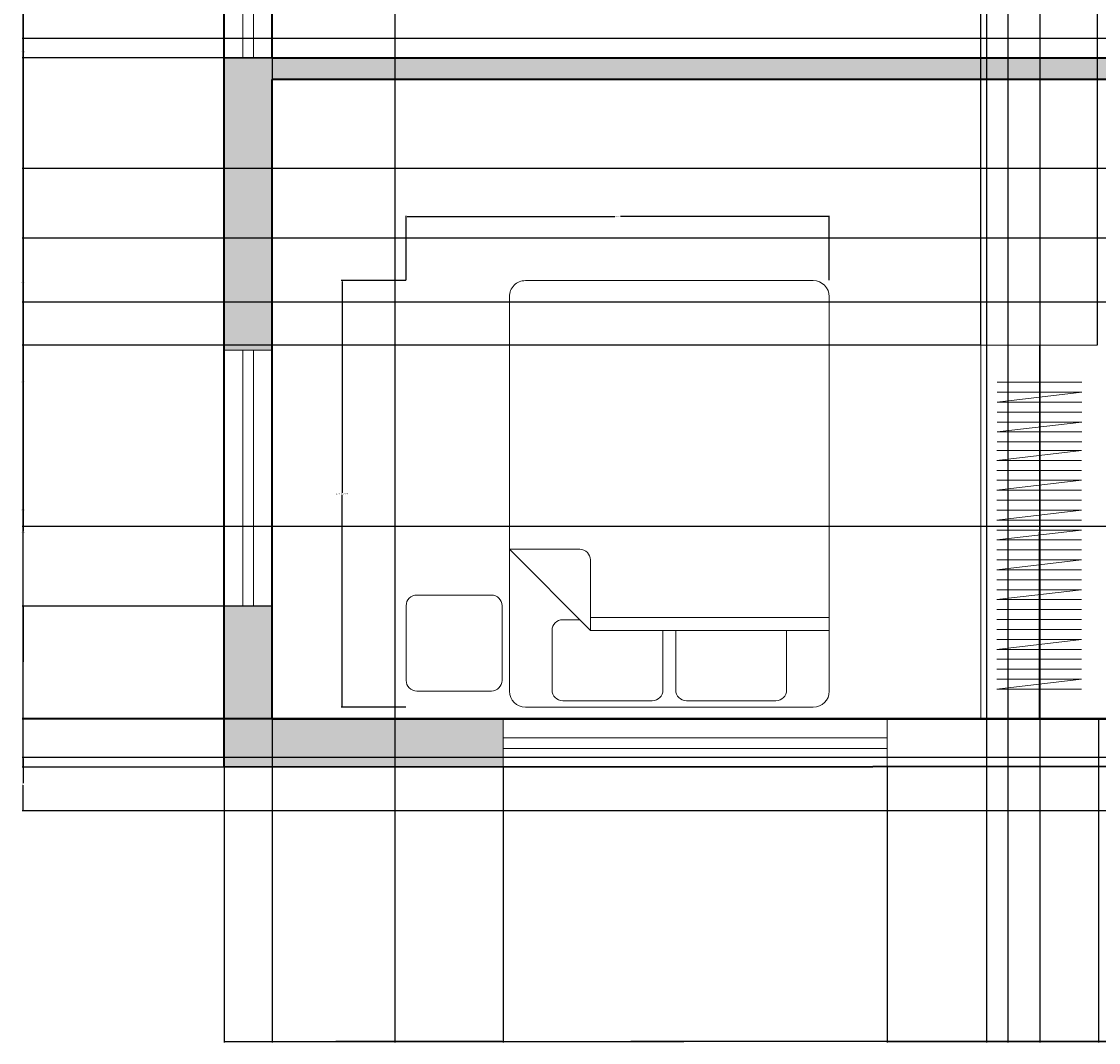
# Model space of a CAD drawing. Units: inches. Extents: x 1531 to 2263, y 2711 to 3216.
# Tile 1 of 12: x 1531 to 1733, y 2711 to 2903. Entities that reach past the tile are written whole.
import ezdxf

# ---------------------------------------------------------------- set-up
doc = ezdxf.new("R2010")
doc.units = ezdxf.units.IN
for name, color, linetype, lineweight in [('A-ANNO-DIMS', 2, 'Continuous', 18), ('A-FLOR-CASE', 9, 'Continuous', 18), ('A-FURN', 8, 'Continuous', 18), ('A-GLAZ', 4, 'Continuous', 18), ('A-WALL', 7, 'Continuous', 35)]:
    doc.layers.add(name, color=color, linetype=linetype, lineweight=lineweight)
doc.layers.add('A-WALL-PATT', color=18, linetype='Continuous', lineweight=13, true_color=0x000000)
doc.styles.get("Standard").update_dxf_attribs({"font": 'arial.ttf'})
doc.dimstyles.get("Standard").update_dxf_attribs({"dimtxt": 0.18, "dimasz": 0.18, "dimexe": 0.18, "dimexo": 0.0625, "dimgap": 0.09, "dimtad": 0, "dimtih": 1, "dimtoh": 1, "dimdec": 4, "dimzin": 0, "dimdsep": 46, "dimtxsty": 'Standard', "dimcen": 0.09, "dimadec": 0, "dimazin": 0, "dimtfac": 1, "dimtdec": 4, "dimtofl": 0, "dimtmove": 0, "dimatfit": 3, "dimfxl": 1, "dimtolj": 1, "dimtzin": 0, "dimarcsym": 0})

# ---------------------------------------------------------------- blocks, each defined once
blk = doc.blocks.new('Bed - Queen')
for p, q in [((3, 0), (57, 0)), ((10, -1.2), (26.8, -1.2)), ((33.2, -1.2), (50, -1.2)), ((0, -77), (0, -3)), ((8, -14.4), (8, -3.2)), ((28.8, -3.2), (28.8, -14.4)), ((31.2, -14.4), (31.2, -3.2)), ((52, -3.2), (52, -14.4)), ((60, -3), (60, -77)), ((0, -14.4), (44.8, -14.4)), ((60, -29.6), (44.8, -14.4)), ((44.8, -14.4), (44.8, -27.6)), ((44.8, -16.8), (0, -16.8)), ((50, -16.4), (46.8, -16.4)), ((46.8, -29.6), (60, -29.6)), ((57, -80), (3, -80))]:
    blk.add_line(p, q)
blk.add_lwpolyline([(63.37, -3.02), (77.37, -3.02, -0.414214), (79.37, -5.02), (79.37, -19.02, -0.414214), (77.37, -21.02), (63.37, -21.02, -0.414214), (61.37, -19.02), (61.37, -5.02, -0.414214)], format="xyb", close=True)
for centre, radius, start, end in [((3, -3), 3, 90, 180), ((57, -3), 3, 0, 90), ((10, -3.2), 2, 90, 180), ((26.8, -3.2), 2, 0, 90), ((33.2, -3.2), 2, 90, 180), ((50, -3.2), 2, 0, 90), ((50, -14.4), 2, 270, 0), ((46.8, -27.6), 2, 180, 270), ((3, -77), 3, 180, 270), ((57, -77), 3, 270, 0)]:
    blk.add_arc(centre, radius, start, end)
blk = doc.blocks.new('WIN-72IN')
for p, q in [((0, 5.5), (72, 5.5)), ((0, 3.5), (72, 3.5))]:
    blk.add_line(p, q)
for points in [[(0, 9), (0, 0)], [(72, 0), (72, 9)]]:
    blk.add_lwpolyline(points)
blk = doc.blocks.new('WIN-48IN')
for p, q in [((3.5, 48), (3.5, 0)), ((5.5, 48), (5.5, 0))]:
    blk.add_line(p, q)
for points in [[(0, 48), (9, 48)], [(9, 0), (0, 0)]]:
    blk.add_lwpolyline(points)
blk = doc.blocks.new('*D32')
at = {"layer": 'A-ANNO-DIMS', "color": 0, "lineweight": -2, "transparency": 16777216}
for p, q in [((1602.99, 2853.97), (1590.87, 2853.97)), ((1591.05, 2853.79), (1591.05, 2814.16)), ((1591.05, 2774.15), (1591.05, 2813.78)), ((1602.99, 2773.97), (1590.87, 2773.97))]:
    blk.add_line(p, q, dxfattribs=at)
at = {"layer": 'A-ANNO-DIMS', "color": 0, "transparency": 16777216}
for points in [[(1591.02, 2853.79), (1591.08, 2853.79), (1591.05, 2853.97)], [(1591.02, 2774.15), (1591.08, 2774.15), (1591.05, 2773.97)]]:
    blk.add_solid(points, dxfattribs=at)
at = {"layer": 'Defpoints', "color": 0, "transparency": 16777216}
for p in [(1603.05, 2853.97), (1591.05, 2773.97), (1603.05, 2773.97)]:
    blk.add_point(p, dxfattribs=at)
at = {"layer": 'A-ANNO-DIMS', "color": 0, "transparency": 16777216, "insert": (1591.05, 2813.97), "char_height": 0.18, "attachment_point": 5}
blk.add_mtext('\\A1;QUEEN BED 80 TYP.', dxfattribs=at)
blk = doc.blocks.new('*D33')
at = {"layer": 'A-ANNO-DIMS', "color": 0, "lineweight": -2, "transparency": 16777216}
for p, q in [((1603.05, 2854.03), (1603.05, 2866.15)), ((1603.23, 2865.97), (1642.21, 2865.97)), ((1682.25, 2865.97), (1643.27, 2865.97)), ((1682.43, 2854.03), (1682.43, 2866.15))]:
    blk.add_line(p, q, dxfattribs=at)
at = {"layer": 'A-ANNO-DIMS', "color": 0, "transparency": 16777216}
for points in [[(1603.23, 2866), (1603.23, 2865.94), (1603.05, 2865.97)], [(1682.25, 2866), (1682.25, 2865.94), (1682.43, 2865.97)]]:
    blk.add_solid(points, dxfattribs=at)
at = {"layer": 'Defpoints', "color": 0, "transparency": 16777216}
for p in [(1603.05, 2865.97), (1603.05, 2853.97), (1682.43, 2853.97)]:
    blk.add_point(p, dxfattribs=at)
at = {"layer": 'A-ANNO-DIMS', "color": 0, "transparency": 16777216, "insert": (1642.74, 2865.97), "char_height": 0.18, "attachment_point": 5}
blk.add_mtext('\\A1;79 TYP.', dxfattribs=at)
blk = doc.blocks.new('*D56')
at = {"layer": 'A-ANNO-DIMS', "color": 0, "lineweight": -2, "transparency": 16777216}
for p, q in [((1568.85, 3182.67), (1531.04, 3182.67)), ((1531.22, 3182.49), (1531.22, 2972.86)), ((1531.22, 2762.85), (1531.22, 2972.49)), ((1568.85, 2762.67), (1531.04, 2762.67))]:
    blk.add_line(p, q, dxfattribs=at)
at = {"layer": 'A-ANNO-DIMS', "color": 0, "transparency": 16777216}
for points in [[(1531.19, 3182.49), (1531.25, 3182.49), (1531.22, 3182.67)], [(1531.19, 2762.85), (1531.25, 2762.85), (1531.22, 2762.67)]]:
    blk.add_solid(points, dxfattribs=at)
at = {"layer": 'Defpoints', "color": 0, "transparency": 16777216}
for p in [(1568.91, 3182.67), (1531.22, 2762.67), (1568.91, 2762.67)]:
    blk.add_point(p, dxfattribs=at)
at = {"layer": 'A-ANNO-DIMS', "color": 0, "transparency": 16777216, "insert": (1531.22, 2972.67), "char_height": 0.18, "attachment_point": 5}
blk.add_mtext('\\A1;420', dxfattribs=at)
blk = doc.blocks.new('*D57')
at = {"layer": 'A-ANNO-DIMS', "color": 0, "lineweight": -2, "transparency": 16777216}
for p, q in [((1577.91, 3029.62), (1577.91, 2711.06)), ((1711.91, 3029.69), (1711.91, 2711.06)), ((1578.09, 2711.24), (1644.63, 2711.24)), ((1711.73, 2711.24), (1645.19, 2711.24))]:
    blk.add_line(p, q, dxfattribs=at)
at = {"layer": 'A-ANNO-DIMS', "color": 0, "transparency": 16777216}
for points in [[(1578.09, 2711.27), (1578.09, 2711.21), (1577.91, 2711.24)], [(1711.73, 2711.27), (1711.73, 2711.21), (1711.91, 2711.24)]]:
    blk.add_solid(points, dxfattribs=at)
at = {"layer": 'Defpoints', "color": 0, "transparency": 16777216}
for p in [(1577.91, 3029.68), (1711.91, 3029.75), (1711.91, 2711.24)]:
    blk.add_point(p, dxfattribs=at)
at = {"layer": 'A-ANNO-DIMS', "color": 0, "transparency": 16777216, "insert": (1644.91, 2711.24), "char_height": 0.18, "attachment_point": 5}
blk.add_mtext('\\A1;134', dxfattribs=at)
blk = doc.blocks.new('*D58')
at = {"layer": 'A-ANNO-DIMS', "color": 0, "lineweight": -2, "transparency": 16777216}
for p, q in [((1715.91, 3097.69), (1715.91, 2711.06)), ((1775.91, 3097.72), (1775.91, 2711.06)), ((1716.09, 2711.24), (1745.69, 2711.24)), ((1775.73, 2711.24), (1746.13, 2711.24))]:
    blk.add_line(p, q, dxfattribs=at)
at = {"layer": 'A-ANNO-DIMS', "color": 0, "transparency": 16777216}
for points in [[(1716.09, 2711.27), (1716.09, 2711.21), (1715.91, 2711.24)], [(1775.73, 2711.27), (1775.73, 2711.21), (1775.91, 2711.24)]]:
    blk.add_solid(points, dxfattribs=at)
at = {"layer": 'Defpoints', "color": 0, "transparency": 16777216}
for p in [(1715.91, 3097.75), (1775.91, 3097.78), (1775.91, 2711.24)]:
    blk.add_point(p, dxfattribs=at)
at = {"layer": 'A-ANNO-DIMS', "color": 0, "transparency": 16777216, "insert": (1745.91, 2711.24), "char_height": 0.18, "attachment_point": 5}
blk.add_mtext('\\A1;60', dxfattribs=at)
blk = doc.blocks.new('*D64')
at = {"layer": 'A-ANNO-DIMS', "color": 0, "lineweight": -2, "transparency": 16777216}
for p, q in [((1779.85, 3025.79), (1531.04, 3025.79)), ((1531.22, 3025.61), (1531.22, 2960.97)), ((1531.22, 2895.96), (1531.22, 2960.6)), ((1775.85, 2895.78), (1531.04, 2895.78))]:
    blk.add_line(p, q, dxfattribs=at)
at = {"layer": 'A-ANNO-DIMS', "color": 0, "transparency": 16777216}
for points in [[(1531.19, 3025.61), (1531.25, 3025.61), (1531.22, 3025.79)], [(1531.19, 2895.96), (1531.25, 2895.96), (1531.22, 2895.78)]]:
    blk.add_solid(points, dxfattribs=at)
at = {"layer": 'Defpoints', "color": 0, "transparency": 16777216}
for p in [(1779.91, 3025.79), (1531.22, 2895.78), (1775.91, 2895.78)]:
    blk.add_point(p, dxfattribs=at)
at = {"layer": 'A-ANNO-DIMS', "color": 0, "transparency": 16777216, "insert": (1531.22, 2960.78), "char_height": 0.18, "attachment_point": 5}
blk.add_mtext('\\A1;130', dxfattribs=at)
blk = doc.blocks.new('*D65')
at = {"layer": 'A-ANNO-DIMS', "color": 0, "lineweight": -2, "transparency": 16777216}
for p, q in [((1577.97, 2891.68), (2262.37, 2891.68)), ((2262.19, 2891.5), (2262.19, 2831.86)), ((2262.19, 2771.86), (2262.19, 2831.5)), ((1577.97, 2771.68), (2262.37, 2771.68))]:
    blk.add_line(p, q, dxfattribs=at)
at = {"layer": 'A-ANNO-DIMS', "color": 0, "transparency": 16777216}
for points in [[(2262.16, 2891.5), (2262.22, 2891.5), (2262.19, 2891.68)], [(2262.16, 2771.86), (2262.22, 2771.86), (2262.19, 2771.68)]]:
    blk.add_solid(points, dxfattribs=at)
at = {"layer": 'Defpoints', "color": 0, "transparency": 16777216}
for p in [(1577.91, 2891.68), (1577.91, 2771.68), (2262.19, 2771.68)]:
    blk.add_point(p, dxfattribs=at)
at = {"layer": 'A-ANNO-DIMS', "color": 0, "transparency": 16777216, "insert": (2262.19, 2831.68), "char_height": 0.18, "attachment_point": 5}
blk.add_mtext('\\A1;120', dxfattribs=at)
blk = doc.blocks.new('*D66')
at = {"layer": 'A-ANNO-DIMS', "color": 0, "lineweight": -2, "transparency": 16777216}
for p, q in [((1577.91, 2895.74), (1577.91, 3216.47)), ((1578.09, 3216.29), (1676.63, 3216.29)), ((1775.73, 3216.29), (1677.19, 3216.29)), ((1775.91, 2895.85), (1775.91, 3216.47))]:
    blk.add_line(p, q, dxfattribs=at)
at = {"layer": 'A-ANNO-DIMS', "color": 0, "transparency": 16777216}
for points in [[(1578.09, 3216.32), (1578.09, 3216.26), (1577.91, 3216.29)], [(1775.73, 3216.32), (1775.73, 3216.26), (1775.91, 3216.29)]]:
    blk.add_solid(points, dxfattribs=at)
at = {"layer": 'Defpoints', "color": 0, "transparency": 16777216}
for p in [(1775.91, 3216.29), (1577.91, 2895.68), (1775.91, 2895.78)]:
    blk.add_point(p, dxfattribs=at)
at = {"layer": 'A-ANNO-DIMS', "color": 0, "transparency": 16777216, "insert": (1676.91, 3216.29), "char_height": 0.18, "attachment_point": 5}
blk.add_mtext('\\A1;198', dxfattribs=at)
blk = doc.blocks.new('*D67')
at = {"layer": 'A-ANNO-DIMS', "color": 0, "lineweight": -2, "transparency": 16777216}
for p, q in [((1577.91, 2771.62), (1577.91, 2711.06)), ((1732.91, 2771.7), (1732.91, 2711.06)), ((1578.09, 2711.24), (1655.13, 2711.24)), ((1732.73, 2711.24), (1655.69, 2711.24))]:
    blk.add_line(p, q, dxfattribs=at)
at = {"layer": 'A-ANNO-DIMS', "color": 0, "transparency": 16777216}
for points in [[(1578.09, 2711.27), (1578.09, 2711.21), (1577.91, 2711.24)], [(1732.73, 2711.27), (1732.73, 2711.21), (1732.91, 2711.24)]]:
    blk.add_solid(points, dxfattribs=at)
at = {"layer": 'Defpoints', "color": 0, "transparency": 16777216}
for p in [(1577.91, 2771.68), (1732.91, 2771.76), (1732.91, 2711.24)]:
    blk.add_point(p, dxfattribs=at)
at = {"layer": 'A-ANNO-DIMS', "color": 0, "transparency": 16777216, "insert": (1655.41, 2711.24), "char_height": 0.18, "attachment_point": 5}
blk.add_mtext('\\A1;155', dxfattribs=at)
blk = doc.blocks.new('*D75')
at = {"layer": 'A-ANNO-DIMS', "color": 0, "lineweight": -2, "transparency": 16777216}
for p, q in [((2219.85, 2899.4), (1531.04, 2899.4)), ((1531.22, 2899.22), (1531.22, 2853.81)), ((1531.22, 2808.04), (1531.22, 2853.45)), ((2219.85, 2807.86), (1531.04, 2807.86))]:
    blk.add_line(p, q, dxfattribs=at)
at = {"layer": 'A-ANNO-DIMS', "color": 0, "transparency": 16777216}
for points in [[(1531.19, 2899.22), (1531.25, 2899.22), (1531.22, 2899.4)], [(1531.19, 2808.04), (1531.25, 2808.04), (1531.22, 2807.86)]]:
    blk.add_solid(points, dxfattribs=at)
at = {"layer": 'Defpoints', "color": 0, "transparency": 16777216}
for p in [(1531.22, 2899.4), (2219.91, 2899.4), (2219.91, 2807.86)]:
    blk.add_point(p, dxfattribs=at)
at = {"layer": 'A-ANNO-DIMS', "color": 0, "transparency": 16777216, "insert": (1531.22, 2853.63), "char_height": 0.18, "attachment_point": 5}
blk.add_mtext('\\A1;91.53', dxfattribs=at)
blk = doc.blocks.new('*D87')
at = {"layer": 'A-ANNO-DIMS', "color": 0, "lineweight": -2, "transparency": 16777216}
for p, q in [((1721.91, 3101.69), (1721.91, 2711.06)), ((1745.91, 3101.7), (1745.91, 2711.06)), ((1722.09, 2711.24), (1733.69, 2711.24)), ((1745.73, 2711.24), (1734.13, 2711.24))]:
    blk.add_line(p, q, dxfattribs=at)
at = {"layer": 'A-ANNO-DIMS', "color": 0, "transparency": 16777216}
for points in [[(1722.09, 2711.27), (1722.09, 2711.21), (1721.91, 2711.24)], [(1745.73, 2711.27), (1745.73, 2711.21), (1745.91, 2711.24)]]:
    blk.add_solid(points, dxfattribs=at)
at = {"layer": 'Defpoints', "color": 0, "transparency": 16777216}
for p in [(1721.91, 3101.75), (1745.91, 3101.77), (1745.91, 2711.24)]:
    blk.add_point(p, dxfattribs=at)
at = {"layer": 'A-ANNO-DIMS', "color": 0, "transparency": 16777216, "insert": (1733.91, 2711.24), "char_height": 0.18, "attachment_point": 5}
blk.add_mtext('\\A1;24', dxfattribs=at)
blk = doc.blocks.new('*D93')
at = {"layer": 'A-ANNO-DIMS', "color": 0, "lineweight": -2, "transparency": 16777216}
for p, q in [((1568.91, 2762.61), (1568.91, 2711.06)), ((1621.26, 2762.64), (1621.26, 2711.06)), ((1569.09, 2711.24), (1594.69, 2711.24)), ((1621.08, 2711.24), (1595.48, 2711.24))]:
    blk.add_line(p, q, dxfattribs=at)
at = {"layer": 'A-ANNO-DIMS', "color": 0, "transparency": 16777216}
for points in [[(1569.09, 2711.27), (1569.09, 2711.21), (1568.91, 2711.24)], [(1621.08, 2711.27), (1621.08, 2711.21), (1621.26, 2711.24)]]:
    blk.add_solid(points, dxfattribs=at)
at = {"layer": 'Defpoints', "color": 0, "transparency": 16777216}
for p in [(1568.91, 2762.67), (1621.26, 2762.7), (1621.26, 2711.24)]:
    blk.add_point(p, dxfattribs=at)
at = {"layer": 'A-ANNO-DIMS', "color": 0, "transparency": 16777216, "insert": (1595.09, 2711.24), "char_height": 0.18, "attachment_point": 5}
blk.add_mtext('\\A1;52.35', dxfattribs=at)
blk = doc.blocks.new('*D94')
at = {"layer": 'A-ANNO-DIMS', "color": 0, "lineweight": -2, "transparency": 16777216}
for p, q in [((1693.26, 2762.64), (1693.26, 2711.06)), ((1751.41, 2762.71), (1751.41, 2711.06)), ((1693.44, 2711.24), (1721.94, 2711.24)), ((1751.23, 2711.24), (1722.73, 2711.24))]:
    blk.add_line(p, q, dxfattribs=at)
at = {"layer": 'A-ANNO-DIMS', "color": 0, "transparency": 16777216}
for points in [[(1693.44, 2711.27), (1693.44, 2711.21), (1693.26, 2711.24)], [(1751.23, 2711.27), (1751.23, 2711.21), (1751.41, 2711.24)]]:
    blk.add_solid(points, dxfattribs=at)
at = {"layer": 'Defpoints', "color": 0, "transparency": 16777216}
for p in [(1693.26, 2762.7), (1751.41, 2762.77), (1751.41, 2711.24)]:
    blk.add_point(p, dxfattribs=at)
at = {"layer": 'A-ANNO-DIMS', "color": 0, "transparency": 16777216, "insert": (1722.34, 2711.24), "char_height": 0.18, "attachment_point": 5}
blk.add_mtext('\\A1;58.15', dxfattribs=at)
blk = doc.blocks.new('*D101')
at = {"layer": 'A-ANNO-DIMS', "color": 0, "lineweight": -2, "transparency": 16777216}
for p, q in [((2228.85, 2918.81), (1531.04, 2918.81)), ((1531.22, 2918.63), (1531.22, 2897.08)), ((1531.22, 2875.18), (1531.22, 2896.72)), ((2228.85, 2875), (1531.04, 2875))]:
    blk.add_line(p, q, dxfattribs=at)
at = {"layer": 'A-ANNO-DIMS', "color": 0, "transparency": 16777216}
for points in [[(1531.19, 2918.63), (1531.25, 2918.63), (1531.22, 2918.81)], [(1531.19, 2875.18), (1531.25, 2875.18), (1531.22, 2875)]]:
    blk.add_solid(points, dxfattribs=at)
at = {"layer": 'Defpoints', "color": 0, "transparency": 16777216}
for p in [(2228.91, 2918.81), (1531.22, 2875), (2228.91, 2875)]:
    blk.add_point(p, dxfattribs=at)
at = {"layer": 'A-ANNO-DIMS', "color": 0, "transparency": 16777216, "insert": (1531.22, 2896.9), "char_height": 0.18, "attachment_point": 5}
blk.add_mtext('\\A1;43.81', dxfattribs=at)
blk = doc.blocks.new('*D104')
at = {"layer": 'A-ANNO-DIMS', "color": 0, "lineweight": -2, "transparency": 16777216}
for p, q in [((1577.85, 2792.93), (1531.04, 2792.93)), ((1531.22, 2792.75), (1531.22, 2782.49)), ((1531.22, 2771.86), (1531.22, 2782.12)), ((1577.85, 2771.68), (1531.04, 2771.68))]:
    blk.add_line(p, q, dxfattribs=at)
at = {"layer": 'A-ANNO-DIMS', "color": 0, "transparency": 16777216}
for points in [[(1531.19, 2792.75), (1531.25, 2792.75), (1531.22, 2792.93)], [(1531.19, 2771.86), (1531.25, 2771.86), (1531.22, 2771.68)]]:
    blk.add_solid(points, dxfattribs=at)
at = {"layer": 'Defpoints', "color": 0, "transparency": 16777216}
for p in [(1531.22, 2792.93), (1577.91, 2792.93), (1577.91, 2771.68)]:
    blk.add_point(p, dxfattribs=at)
at = {"layer": 'A-ANNO-DIMS', "color": 0, "transparency": 16777216, "insert": (1531.22, 2782.3), "char_height": 0.18, "attachment_point": 5}
blk.add_mtext('\\A1;21.25', dxfattribs=at)
blk = doc.blocks.new('*D113')
at = {"layer": 'A-ANNO-DIMS', "color": 0, "lineweight": -2, "transparency": 16777216}
for p, q in [((1577.91, 2913.88), (1577.91, 2711.06)), ((1600.94, 2913.88), (1600.94, 2711.06)), ((1578.09, 2711.24), (1588.96, 2711.24)), ((1600.76, 2711.24), (1589.89, 2711.24))]:
    blk.add_line(p, q, dxfattribs=at)
at = {"layer": 'A-ANNO-DIMS', "color": 0, "transparency": 16777216}
for points in [[(1578.09, 2711.27), (1578.09, 2711.21), (1577.91, 2711.24)], [(1600.76, 2711.27), (1600.76, 2711.21), (1600.94, 2711.24)]]:
    blk.add_solid(points, dxfattribs=at)
at = {"layer": 'Defpoints', "color": 0, "transparency": 16777216}
for p in [(1577.91, 2913.94), (1600.94, 2913.94), (1600.94, 2711.24)]:
    blk.add_point(p, dxfattribs=at)
at = {"layer": 'A-ANNO-DIMS', "color": 0, "transparency": 16777216, "insert": (1589.43, 2711.24), "char_height": 0.18, "attachment_point": 5}
blk.add_mtext('\\A1;23.034', dxfattribs=at)
blk = doc.blocks.new('*D114')
at = {"layer": 'A-ANNO-DIMS', "color": 0, "lineweight": -2, "transparency": 16777216}
for p, q in [((1577.97, 2913.94), (2262.37, 2913.94)), ((2262.19, 2913.76), (2262.19, 2904.99)), ((2262.19, 2895.86), (2262.19, 2904.63)), ((1577.97, 2895.68), (2262.37, 2895.68))]:
    blk.add_line(p, q, dxfattribs=at)
at = {"layer": 'A-ANNO-DIMS', "color": 0, "transparency": 16777216}
for points in [[(2262.16, 2913.76), (2262.22, 2913.76), (2262.19, 2913.94)], [(2262.16, 2895.86), (2262.22, 2895.86), (2262.19, 2895.68)]]:
    blk.add_solid(points, dxfattribs=at)
at = {"layer": 'Defpoints', "color": 0, "transparency": 16777216}
for p in [(1577.91, 2913.94), (1577.91, 2895.68), (2262.19, 2895.68)]:
    blk.add_point(p, dxfattribs=at)
at = {"layer": 'A-ANNO-DIMS', "color": 0, "transparency": 16777216, "insert": (2262.19, 2904.81), "char_height": 0.18, "attachment_point": 5}
blk.add_mtext('\\A1;18.26', dxfattribs=at)
blk = doc.blocks.new('*D125')
at = {"layer": 'A-ANNO-DIMS', "color": 0, "lineweight": -2, "transparency": 16777216}
for p, q in [((2076.85, 2861.95), (1531.04, 2861.95)), ((1531.22, 2861.77), (1531.22, 2835.09)), ((1531.22, 2808.04), (1531.22, 2834.72)), ((2076.85, 2807.86), (1531.04, 2807.86))]:
    blk.add_line(p, q, dxfattribs=at)
at = {"layer": 'A-ANNO-DIMS', "color": 0, "transparency": 16777216}
for points in [[(1531.19, 2861.77), (1531.25, 2861.77), (1531.22, 2861.95)], [(1531.19, 2808.04), (1531.25, 2808.04), (1531.22, 2807.86)]]:
    blk.add_solid(points, dxfattribs=at)
at = {"layer": 'Defpoints', "color": 0, "transparency": 16777216}
for p in [(2076.91, 2861.95), (1531.22, 2807.86), (2076.91, 2807.86)]:
    blk.add_point(p, dxfattribs=at)
at = {"layer": 'A-ANNO-DIMS', "color": 0, "transparency": 16777216, "insert": (1531.22, 2834.91), "char_height": 0.18, "attachment_point": 5}
blk.add_mtext('\\A1;54.09', dxfattribs=at)
blk = doc.blocks.new('*D127')
at = {"layer": 'A-ANNO-DIMS', "color": 0, "lineweight": -2, "transparency": 16777216}
for p, q in [((1902.92, 2849.94), (1531.04, 2849.94)), ((1531.22, 2849.76), (1531.22, 2811.07)), ((1531.22, 2772.03), (1531.22, 2810.71)), ((1902.92, 2771.85), (1531.04, 2771.85))]:
    blk.add_line(p, q, dxfattribs=at)
at = {"layer": 'A-ANNO-DIMS', "color": 0, "transparency": 16777216}
for points in [[(1531.19, 2849.76), (1531.25, 2849.76), (1531.22, 2849.94)], [(1531.19, 2772.03), (1531.25, 2772.03), (1531.22, 2771.85)]]:
    blk.add_solid(points, dxfattribs=at)
at = {"layer": 'Defpoints', "color": 0, "transparency": 16777216}
for p in [(1902.99, 2849.94), (1531.22, 2771.85), (1902.99, 2771.85)]:
    blk.add_point(p, dxfattribs=at)
at = {"layer": 'A-ANNO-DIMS', "color": 0, "transparency": 16777216, "insert": (1531.22, 2810.89), "char_height": 0.18, "attachment_point": 5}
blk.add_mtext('\\A1;78.09', dxfattribs=at)
blk = doc.blocks.new('*D128')
at = {"layer": 'A-ANNO-DIMS', "color": 0, "lineweight": -2, "transparency": 16777216}
for p, q in [((1710.84, 2841.9), (1710.84, 3216.47)), ((1711.02, 3216.29), (1721.3, 3216.29)), ((1732.52, 3216.29), (1722.23, 3216.29)), ((1732.7, 2841.9), (1732.7, 3216.47))]:
    blk.add_line(p, q, dxfattribs=at)
at = {"layer": 'A-ANNO-DIMS', "color": 0, "transparency": 16777216}
for points in [[(1711.02, 3216.32), (1711.02, 3216.26), (1710.84, 3216.29)], [(1732.52, 3216.32), (1732.52, 3216.26), (1732.7, 3216.29)]]:
    blk.add_solid(points, dxfattribs=at)
at = {"layer": 'Defpoints', "color": 0, "transparency": 16777216}
for p in [(1732.7, 3216.29), (1710.84, 2841.84), (1732.7, 2841.84)]:
    blk.add_point(p, dxfattribs=at)
at = {"layer": 'A-ANNO-DIMS', "color": 0, "transparency": 16777216, "insert": (1721.77, 3216.29), "char_height": 0.18, "attachment_point": 5}
blk.add_mtext('\\A1;21.866', dxfattribs=at)
blk = doc.blocks.new('*D129')
at = {"layer": 'A-ANNO-DIMS', "color": 0, "lineweight": -2, "transparency": 16777216}
for p, q in [((1710.77, 2841.84), (1531.04, 2841.84)), ((1531.22, 2841.66), (1531.22, 2806.97)), ((1531.22, 2771.93), (1531.22, 2806.61)), ((1710.77, 2771.75), (1531.04, 2771.75))]:
    blk.add_line(p, q, dxfattribs=at)
at = {"layer": 'A-ANNO-DIMS', "color": 0, "transparency": 16777216}
for points in [[(1531.19, 2841.66), (1531.25, 2841.66), (1531.22, 2841.84)], [(1531.19, 2771.93), (1531.25, 2771.93), (1531.22, 2771.75)]]:
    blk.add_solid(points, dxfattribs=at)
at = {"layer": 'Defpoints', "color": 0, "transparency": 16777216}
for p in [(1710.84, 2841.84), (1531.22, 2771.75), (1710.84, 2771.75)]:
    blk.add_point(p, dxfattribs=at)
at = {"layer": 'A-ANNO-DIMS', "color": 0, "transparency": 16777216, "insert": (1531.22, 2806.79), "char_height": 0.18, "attachment_point": 5}
blk.add_mtext('\\A1;70.09', dxfattribs=at)
blk = doc.blocks.new('*D131')
at = {"layer": 'A-ANNO-DIMS', "color": 0, "lineweight": -2, "transparency": 16777216}
for p, q in [((1986.59, 2764.52), (1531.04, 2764.52)), ((1531.22, 2764.34), (1531.22, 2759.7)), ((1531.22, 2754.7), (1531.22, 2759.33)), ((1986.59, 2754.52), (1531.04, 2754.52))]:
    blk.add_line(p, q, dxfattribs=at)
at = {"layer": 'A-ANNO-DIMS', "color": 0, "transparency": 16777216}
for points in [[(1531.19, 2764.34), (1531.25, 2764.34), (1531.22, 2764.52)], [(1531.19, 2754.7), (1531.25, 2754.7), (1531.22, 2754.52)]]:
    blk.add_solid(points, dxfattribs=at)
at = {"layer": 'Defpoints', "color": 0, "transparency": 16777216}
for p in [(1531.22, 2764.52), (1986.65, 2764.52), (1986.65, 2754.52)]:
    blk.add_point(p, dxfattribs=at)
at = {"layer": 'A-ANNO-DIMS', "color": 0, "transparency": 16777216, "insert": (1531.22, 2759.52), "char_height": 0.18, "attachment_point": 5}
blk.add_mtext('\\A1;10', dxfattribs=at)

msp = doc.modelspace()

# ---------------------------------------------------------------- hatches: boundary and pattern name
at = {"layer": 'A-WALL-PATT'}
h = msp.add_hatch(color=256, dxfattribs=at)
h.dxf.hatch_style = 1
h.paths.add_polyline_path([(1577.9111, 2891.6796), (1779.9101, 2891.7852), (1779.9101, 2895.7852), (1779.9101, 2901.7852), (1775.9101, 2901.7831), (1775.9101, 2895.7831), (1577.8462, 2895.6795), (1568.9111, 2895.6795), (1568.9111, 2840.9289), (1577.9111, 2840.9289)])
h = msp.add_hatch(color=256, dxfattribs=at)
h.dxf.hatch_style = 1
h.paths.add_polyline_path([(1621.2627, 2771.7022), (1577.9111, 2771.6796), (1577.9111, 2792.9289), (1568.9111, 2792.9289), (1568.9111, 2762.6748), (1621.2627, 2762.7022)])

# ---------------------------------------------------------------- linework, layer by layer
at = {"layer": 'A-FLOR-CASE'}
for p, q in [((1710.8363, 2841.8359), (1732.7021, 2841.8359)), ((1710.8363, 2841.8359), (1710.8363, 2825.8359)), ((1721.8562, 2841.8359), (1721.7692, 2771.7491)), ((1713.9054, 2834.9044), (1729.7712, 2834.9044)), ((1713.9054, 2833.0392), (1729.7712, 2833.0392)), ((1729.7712, 2833.0392), (1713.9054, 2831.1741)), ((1713.9054, 2831.1741), (1729.7712, 2831.1741)), ((1713.9054, 2829.309), (1729.7712, 2829.309)), ((1713.9054, 2827.4438), (1729.7712, 2827.4438)), ((1729.7712, 2827.4438), (1713.9054, 2825.5787)), ((1710.8311, 2823.9708), (1710.8363, 2823.9708)), ((1710.8363, 2825.8359), (1710.8363, 2771.7491)), ((1710.8363, 2771.7491), (1710.8363, 2825.8359)), ((1713.9054, 2825.5787), (1729.7712, 2825.5787)), ((1710.826, 2822.1056), (1710.8363, 2822.1056)), ((1713.8363, 2822.1056), (1729.7021, 2822.1056)), ((1729.7021, 2822.1056), (1713.8363, 2820.2405)), ((1713.9054, 2823.7136), (1729.7712, 2823.7136)), ((1710.8208, 2820.2405), (1710.8363, 2820.2405)), ((1713.8363, 2820.2405), (1729.7021, 2820.2405)), ((1713.8363, 2818.3754), (1729.7021, 2818.3754)), ((1713.8363, 2816.5102), (1729.7021, 2816.5102)), ((1729.7021, 2816.5102), (1713.8363, 2814.6451)), ((1713.8363, 2814.6451), (1729.7021, 2814.6451)), ((1713.8363, 2812.78), (1729.7021, 2812.78)), ((1713.8363, 2810.9148), (1729.7021, 2810.9148)), ((1729.7021, 2810.9148), (1713.8363, 2809.0497)), ((1713.8363, 2809.0497), (1729.7021, 2809.0497)), ((1713.8363, 2807.1845), (1729.7021, 2807.1845)), ((1729.7021, 2807.1845), (1713.8363, 2805.3194)), ((1713.8363, 2805.3194), (1729.7021, 2805.3194)), ((1713.8363, 2803.4543), (1729.7021, 2803.4543)), ((1713.8363, 2801.5891), (1729.7021, 2801.5891)), ((1729.7021, 2801.5891), (1713.8363, 2799.724)), ((1713.8363, 2799.724), (1729.7021, 2799.724)), ((1713.8363, 2797.8589), (1729.7021, 2797.8589)), ((1713.8363, 2795.9937), (1729.7021, 2795.9937)), ((1729.7021, 2795.9937), (1713.8363, 2794.1286)), ((1713.8363, 2794.1286), (1729.7021, 2794.1286)), ((1713.8363, 2792.2635), (1729.7021, 2792.2635)), ((1713.8363, 2790.3983), (1729.7021, 2790.3983)), ((1713.8363, 2788.5332), (1729.7021, 2788.5332)), ((1713.8363, 2786.6681), (1729.7021, 2786.6681)), ((1729.7021, 2786.6681), (1713.8363, 2784.8029)), ((1713.8363, 2784.8029), (1729.7021, 2784.8029)), ((1713.8363, 2782.9378), (1729.7021, 2782.9378)), ((1713.8363, 2781.0727), (1729.7021, 2781.0727)), ((1713.8363, 2779.2075), (1729.7021, 2779.2075)), ((1729.7021, 2779.2075), (1713.8363, 2777.3424)), ((1713.8363, 2777.3424), (1729.7021, 2777.3424)), ((1732.7021, 2771.7491), (1710.8363, 2771.7491))]:
    msp.add_line(p, q, dxfattribs=at)
at = {"layer": 'A-GLAZ'}
for p, q in [((1572.4111, 2953.6795), (1572.4111, 2895.6795)), ((1574.4111, 2953.6795), (1574.4111, 2895.6795)), ((1577.8462, 2895.6795), (1568.9111, 2895.6795))]:
    msp.add_line(p, q, dxfattribs=at)
at = {"layer": 'A-WALL'}
for p, q in [((1577.9111, 2895.6796), (1577.9111, 3025.6795)), ((1775.9101, 2895.7831), (1577.8462, 2895.6795)), ((1779.9101, 2891.7852), (1577.8483, 2891.6795)), ((1577.9111, 2771.6796), (1577.9111, 2891.6796)), ((1577.9111, 2843.6796), (1577.8734, 2843.6795)), ((1732.9101, 2771.7606), (1577.9111, 2771.6796))]:
    msp.add_line(p, q, dxfattribs=at)
msp.add_lwpolyline([(1933.9101, 2762.8657), (1568.9111, 2762.6748), (1568.9111, 3182.6749), (2228.9101, 3183.02), (2228.9101, 2798.8631)], dxfattribs=at)

# ---------------------------------------------------------------- block references
at = {"layer": 'A-FURN', "rotation": 180}
msp.add_blockref('Bed - Queen', (1682.4258, 2773.9664), dxfattribs=at)
at = {"layer": 'A-GLAZ'}
for name, p in [('WIN-48IN', (1568.911, 2792.9294)), ('WIN-72IN', (1621.2628, 2762.7022))]:
    msp.add_blockref(name, p, dxfattribs=at)

# ---------------------------------------------------------------- dimensions: what is measured, and where the dimension line sits
at = {"layer": 'A-ANNO-DIMS'}
for base, p1, p2, override, picture, middle in [((1775.9101, 3216.295), (1577.9111, 2895.6796), (1775.9101, 2895.7831), {"dimdec": 0, "dimlfac": 1, "dimrnd": 0, "dimzin": 0, "dimdsep": 46, "dimlunit": 2}, '*D66', (1676.9106, 3216.295)), ((1732.7021, 3216.295), (1710.8363, 2841.8359), (1732.7021, 2841.8359), {"dimdec": 3, "dimlfac": 1, "dimrnd": 0, "dimzin": 0, "dimdsep": 46, "dimlunit": 2}, '*D128', (1721.7692, 3216.295)), ((1745.9101, 2711.2407), (1721.9101, 3101.7549), (1745.9101, 3101.7674), {"dimdec": 0, "dimlfac": 1, "dimrnd": 0, "dimzin": 0, "dimdsep": 46, "dimlunit": 2}, '*D87', (1733.9101, 2711.2407)), ((1775.9101, 2711.2407), (1715.9101, 3097.7517), (1775.9101, 3097.7831), {"dimdec": 0, "dimlfac": 1, "dimrnd": 0, "dimzin": 0, "dimdsep": 46, "dimlunit": 2}, '*D58', (1745.9101, 2711.2407)), ((1711.9101, 2711.2407), (1577.9111, 3029.6795), (1711.9101, 3029.7496), {"dimdec": 0, "dimlfac": 1, "dimrnd": 0, "dimzin": 0, "dimdsep": 46, "dimlunit": 2}, '*D57', (1644.9106, 2711.2407)), ((1600.9446, 2711.24067), (1577.91107, 2913.93777), (1600.9446, 2913.93777), {"dimdec": 3, "dimlfac": 1, "dimrnd": 0, "dimzin": 0, "dimdsep": 46, "dimlunit": 2}, '*D113', (1589.42783, 2711.24067)), ((1732.9101, 2711.2407), (1577.9111, 2771.6796), (1732.9101, 2771.7606), {"dimdec": 0, "dimlfac": 1, "dimrnd": 0, "dimzin": 0, "dimdsep": 46, "dimlunit": 2}, '*D67', (1655.4106, 2711.2407)), ((1621.2627, 2711.2407), (1568.9111, 2762.6748), (1621.2627, 2762.7022), {"dimdec": 2, "dimlfac": 1, "dimrnd": 0, "dimzin": 0, "dimdsep": 46, "dimlunit": 2}, '*D93', (1595.0869, 2711.2407)), ((1751.4106, 2711.2407), (1693.2627, 2762.7022), (1751.4106, 2762.7703), {"dimdec": 2, "dimlfac": 1, "dimrnd": 0, "dimzin": 0, "dimdsep": 46, "dimlunit": 2}, '*D94', (1722.3367, 2711.2407))]:
    dim = msp.add_linear_dim(base=base, p1=p1, p2=p2, dimstyle='Standard', override=override, dxfattribs=at)
    dim.commit()
    dim.dimension.update_dxf_attribs({"geometry": picture, "text_midpoint": middle})
for base, p1, p2, override, picture, middle in [((1531.2212, 2762.6748), (1568.9111, 3182.6749), (1568.9111, 2762.6748), {"dimdec": 0, "dimlfac": 1, "dimrnd": 0, "dimzin": 0, "dimdsep": 46, "dimlunit": 2}, '*D56', (1531.2212, 2972.6748)), ((1531.2212, 2895.7831), (1779.9101, 3025.7852), (1775.9101, 2895.7831), {"dimdec": 0, "dimlfac": 1, "dimrnd": 0, "dimzin": 0, "dimdsep": 46, "dimlunit": 2}, '*D64', (1531.2212, 2960.7841)), ((1531.2212, 2874.9957), (2228.9101, 2918.8056), (2228.9101, 2874.9957), {"dimdec": 2, "dimlfac": 1, "dimrnd": 0, "dimzin": 0, "dimdsep": 46, "dimlunit": 2}, '*D101', (1531.2212, 2896.9007)), ((2262.1851, 2895.6796), (1577.9111, 2913.9378), (1577.9111, 2895.6796), {"dimdec": 2, "dimlfac": 1, "dimrnd": 0, "dimzin": 0, "dimdsep": 46, "dimlunit": 2}, '*D114', (2262.1851, 2904.8087)), ((1531.2212, 2899.3968), (2219.9101, 2807.8631), (2219.9101, 2899.3968), {"dimdec": 2, "dimlfac": 1, "dimrnd": 0, "dimzin": 0, "dimdsep": 46, "dimlunit": 2}, '*D75', (1531.2212, 2853.63)), ((2262.1851, 2771.6796), (1577.9111, 2891.6796), (1577.9111, 2771.6796), {"dimdec": 0, "dimlfac": 1, "dimrnd": 0, "dimzin": 0, "dimdsep": 46, "dimlunit": 2}, '*D65', (2262.1851, 2831.6796)), ((1531.2212, 2807.8631), (2076.9101, 2861.9499), (2076.9101, 2807.8631), {"dimdec": 2, "dimlfac": 1, "dimrnd": 0, "dimzin": 0, "dimdsep": 46, "dimlunit": 2}, '*D125', (1531.2212, 2834.9065)), ((1531.2212, 2771.8496), (1902.9862, 2849.9364), (1902.9862, 2771.8496), {"dimdec": 2, "dimlfac": 1, "dimrnd": 0, "dimzin": 0, "dimdsep": 46, "dimlunit": 2}, '*D127', (1531.2212, 2810.893)), ((1531.2212, 2771.7491), (1710.8363, 2841.8359), (1710.8363, 2771.7491), {"dimdec": 2, "dimlfac": 1, "dimrnd": 0, "dimzin": 0, "dimdsep": 46, "dimlunit": 2}, '*D129', (1531.2212, 2806.7925)), ((1531.2212, 2792.9289), (1577.9111, 2771.6796), (1577.9111, 2792.9289), {"dimdec": 2, "dimlfac": 1, "dimrnd": 0, "dimzin": 0, "dimdsep": 46, "dimlunit": 2}, '*D104', (1531.2212, 2782.3042)), ((1531.2212, 2764.5157), (1986.6484, 2754.5157), (1986.6484, 2764.5157), {"dimdec": 0, "dimlfac": 1, "dimrnd": 0, "dimzin": 0, "dimdsep": 46, "dimlunit": 2}, '*D131', (1531.2212, 2759.5157))]:
    dim = msp.add_linear_dim(base=base, p1=p1, p2=p2, angle=90, dimstyle='Standard', override=override, dxfattribs=at)
    dim.commit()
    dim.dimension.update_dxf_attribs({"geometry": picture, "text_midpoint": middle})
for base, p1, p2, angle, text, picture, middle in [((1603.0522, 2865.9665), (1682.4258, 2853.9665), (1603.0522, 2853.9665), 180, '<> TYP.', '*D33', (1642.739, 2865.9665)), ((1591.0522, 2773.9664), (1603.0522, 2853.9665), (1603.0522, 2773.9664), 270, 'QUEEN BED <> TYP.', '*D32', (1591.0522, 2813.9664))]:
    dim = msp.add_linear_dim(base=base, p1=p1, p2=p2, angle=angle, text=text, dimstyle='Standard', override={"dimdec": 0, "dimlfac": 1, "dimrnd": 0, "dimzin": 0, "dimdsep": 46, "dimlunit": 2}, dxfattribs=at)
    dim.commit()
    dim.dimension.update_dxf_attribs({"geometry": picture, "text_midpoint": middle})

doc.saveas('drawing.dxf')
